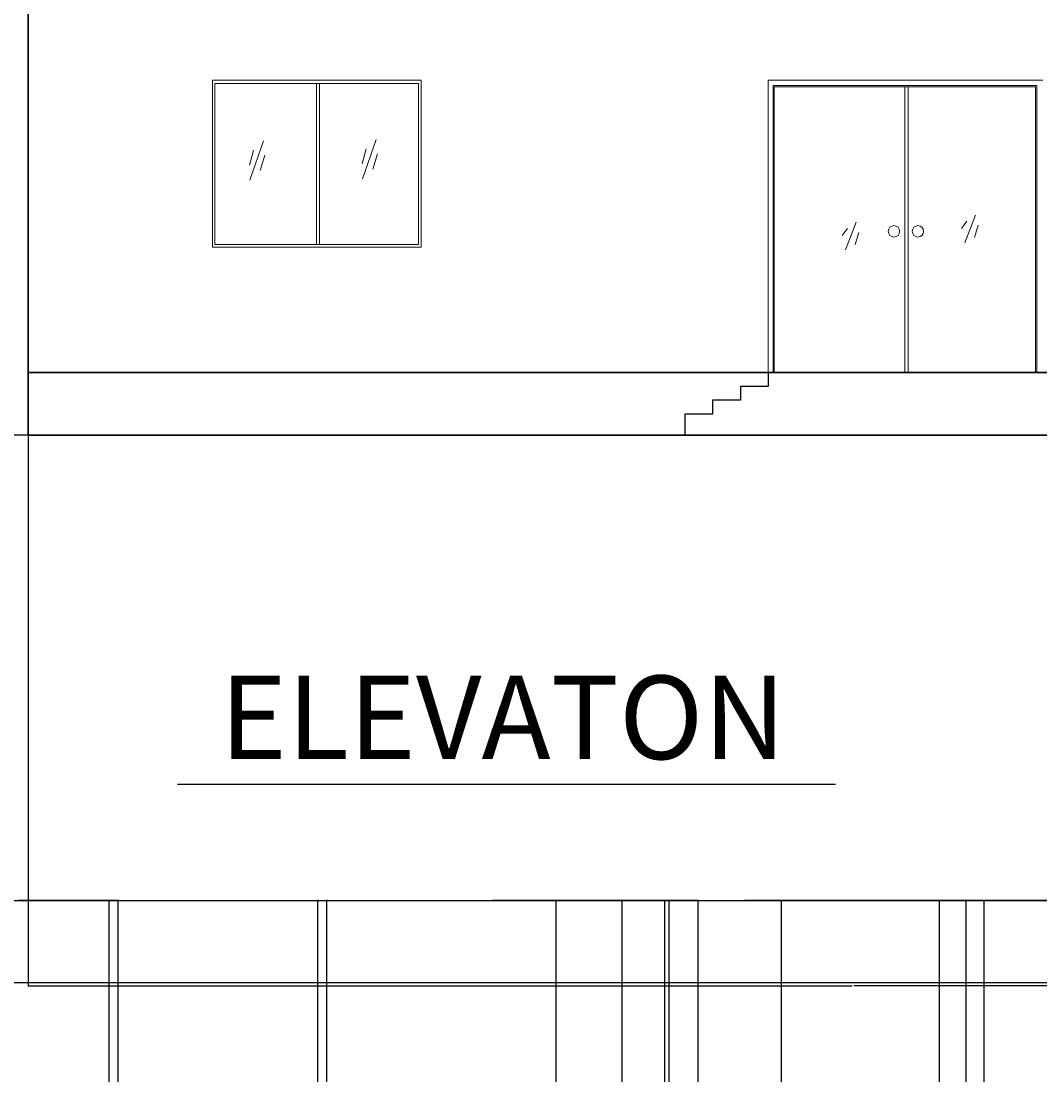
# Model space of a CAD drawing. Units: inches. Extents: x 1770 to 2988, y 1161 to 3221.
# Tile 34 of 44: x 2179 to 2472, y 2520 to 2823. Entities that reach past the tile are written whole.
import ezdxf

# ---------------------------------------------------------------- set-up
doc = ezdxf.new("R2010")
doc.units = ezdxf.units.IN
for name, color, linetype, lineweight in [('A-ANNO-DIMS', 2, 'Continuous', 18), ('A-ANNO-TEXT', 7, 'Continuous', 25), ('A-ANNO-TTLB', 7, 'Continuous', 25), ('A-ELEV', 7, 'Continuous', 35), ('A-ELEV-DOOR', 4, 'Continuous', 18), ('A-ELEV-GLAZ', 4, 'Continuous', 18), ('A-ELEV-STRS', 7, 'Continuous', 25)]:
    doc.layers.add(name, color=color, linetype=linetype, lineweight=lineweight)
doc.styles.get("Standard").update_dxf_attribs({"font": 'arial.ttf'})
doc.dimstyles.get("Standard").update_dxf_attribs({"dimtxt": 0.18, "dimasz": 0.18, "dimexe": 0.18, "dimexo": 0.0625, "dimgap": 0.09, "dimtad": 0, "dimtih": 1, "dimtoh": 1, "dimdec": 4, "dimzin": 0, "dimdsep": 46, "dimtxsty": 'Standard', "dimcen": 0.09, "dimadec": 0, "dimazin": 0, "dimtfac": 1, "dimtdec": 4, "dimtofl": 0, "dimtmove": 0, "dimatfit": 3, "dimfxl": 1, "dimtolj": 1, "dimtzin": 0, "dimarcsym": 0})

# ---------------------------------------------------------------- blocks, each defined once
blk = doc.blocks.new('GLASS-MARK-WINDOW')
for p, q in [((4.02, 11.23), (0.09, 0)), ((1.17, 8.59), (0, 4.27)), ((4.4, 7.13), (3.12, 2.69))]:
    blk.add_line(p, q)
blk = doc.blocks.new('GLASS-MARK-ENTRY')
for p, q in [((1.47, 6.19), (0, 4.09)), ((3.95, 7.93), (0.91, 0)), ((4.77, 5.04), (3.66, 1.5))]:
    blk.add_line(p, q)
blk = doc.blocks.new('*D56')
at = {"layer": 'A-ANNO-DIMS', "color": 0, "lineweight": -2, "transparency": 16777216}
for p, q in [((1971.53, 2506.34), (1971.53, 2570.7)), ((1971.71, 2570.52), (2386.59, 2570.52)), ((2802.26, 2570.52), (2387.38, 2570.52)), ((2802.44, 2506.34), (2802.44, 2570.7))]:
    blk.add_line(p, q, dxfattribs=at)
at = {"layer": 'A-ANNO-DIMS', "color": 0, "transparency": 16777216}
for points in [[(1971.71, 2570.55), (1971.71, 2570.49), (1971.53, 2570.52)], [(2802.26, 2570.55), (2802.26, 2570.49), (2802.44, 2570.52)]]:
    blk.add_solid(points, dxfattribs=at)
at = {"layer": 'Defpoints', "color": 0, "transparency": 16777216}
for p in [(2802.44, 2570.52), (1971.53, 2506.27), (2802.44, 2506.27)]:
    blk.add_point(p, dxfattribs=at)
at = {"layer": 'A-ANNO-DIMS', "color": 0, "transparency": 16777216, "insert": (2386.99, 2570.52), "char_height": 0.18, "attachment_point": 5}
blk.add_mtext('\\A1;830.9', dxfattribs=at)
blk = doc.blocks.new('*D63')
at = {"layer": 'A-ANNO-DIMS', "color": 0, "lineweight": -2, "transparency": 16777216}
for p, q in [((2352.17, 1323.59), (2352.17, 2570.7)), ((2352.35, 2570.52), (2401.24, 2570.52)), ((2450.91, 2570.52), (2402.02, 2570.52)), ((2451.09, 1323.59), (2451.09, 2570.7))]:
    blk.add_line(p, q, dxfattribs=at)
at = {"layer": 'A-ANNO-DIMS', "color": 0, "transparency": 16777216}
for points in [[(2352.35, 2570.55), (2352.35, 2570.49), (2352.17, 2570.52)], [(2450.91, 2570.55), (2450.91, 2570.49), (2451.09, 2570.52)]]:
    blk.add_solid(points, dxfattribs=at)
at = {"layer": 'Defpoints', "color": 0, "transparency": 16777216}
for p in [(2451.09, 2570.52), (2352.17, 1323.53), (2451.09, 1323.53)]:
    blk.add_point(p, dxfattribs=at)
at = {"layer": 'A-ANNO-DIMS', "color": 0, "transparency": 16777216, "insert": (2401.63, 2570.52), "char_height": 0.18, "attachment_point": 5}
blk.add_mtext('\\A1;98.93', dxfattribs=at)
blk = doc.blocks.new('*D64')
at = {"layer": 'A-ANNO-DIMS', "color": 0, "lineweight": -2, "transparency": 16777216}
for p, q in [((2151.7, 2376.76), (2151.7, 2570.7)), ((2151.88, 2570.52), (2179.09, 2570.52)), ((2207.1, 2570.52), (2179.88, 2570.52)), ((2207.28, 2376.76), (2207.28, 2570.7))]:
    blk.add_line(p, q, dxfattribs=at)
at = {"layer": 'A-ANNO-DIMS', "color": 0, "transparency": 16777216}
for points in [[(2151.88, 2570.55), (2151.88, 2570.49), (2151.7, 2570.52)], [(2207.1, 2570.55), (2207.1, 2570.49), (2207.28, 2570.52)]]:
    blk.add_solid(points, dxfattribs=at)
at = {"layer": 'Defpoints', "color": 0, "transparency": 16777216}
for p in [(2207.28, 2570.52), (2151.7, 2376.7), (2207.28, 2376.7)]:
    blk.add_point(p, dxfattribs=at)
at = {"layer": 'A-ANNO-DIMS', "color": 0, "transparency": 16777216, "insert": (2179.49, 2570.52), "char_height": 0.18, "attachment_point": 5}
blk.add_mtext('\\A1;55.58', dxfattribs=at)
blk = doc.blocks.new('*D65')
at = {"layer": 'A-ANNO-DIMS', "color": 0, "lineweight": -2, "transparency": 16777216}
for p, q in [((2267.28, 2376.76), (2267.28, 2570.7)), ((2267.46, 2570.52), (2320.24, 2570.52)), ((2373.79, 2570.52), (2321.01, 2570.52)), ((2373.97, 2376.76), (2373.97, 2570.7))]:
    blk.add_line(p, q, dxfattribs=at)
at = {"layer": 'A-ANNO-DIMS', "color": 0, "transparency": 16777216}
for points in [[(2267.46, 2570.55), (2267.46, 2570.49), (2267.28, 2570.52)], [(2373.79, 2570.55), (2373.79, 2570.49), (2373.97, 2570.52)]]:
    blk.add_solid(points, dxfattribs=at)
at = {"layer": 'Defpoints', "color": 0, "transparency": 16777216}
for p in [(2373.97, 2570.52), (2267.28, 2376.7), (2373.97, 2376.7)]:
    blk.add_point(p, dxfattribs=at)
at = {"layer": 'A-ANNO-DIMS', "color": 0, "transparency": 16777216, "insert": (2320.62, 2570.52), "char_height": 0.18, "attachment_point": 5}
blk.add_mtext('\\A1;106.7', dxfattribs=at)
blk = doc.blocks.new('*D66')
at = {"layer": 'A-ANNO-DIMS', "color": 0, "lineweight": -2, "transparency": 16777216}
for p, q in [((2397.97, 2376.76), (2397.97, 2570.7)), ((2398.15, 2570.52), (2459.91, 2570.52)), ((2522.58, 2570.52), (2460.82, 2570.52)), ((2522.76, 2376.76), (2522.76, 2570.7))]:
    blk.add_line(p, q, dxfattribs=at)
at = {"layer": 'A-ANNO-DIMS', "color": 0, "transparency": 16777216}
for points in [[(2398.15, 2570.55), (2398.15, 2570.49), (2397.97, 2570.52)], [(2522.58, 2570.55), (2522.58, 2570.49), (2522.76, 2570.52)]]:
    blk.add_solid(points, dxfattribs=at)
at = {"layer": 'Defpoints', "color": 0, "transparency": 16777216}
for p in [(2522.76, 2570.52), (2397.97, 2376.7), (2522.76, 2376.7)]:
    blk.add_point(p, dxfattribs=at)
at = {"layer": 'A-ANNO-DIMS', "color": 0, "transparency": 16777216, "insert": (2460.36, 2570.52), "char_height": 0.18, "attachment_point": 5}
blk.add_mtext('\\A1;124.78', dxfattribs=at)
blk = doc.blocks.new('*D68')
at = {"layer": 'A-ANNO-DIMS', "color": 0, "lineweight": -2, "transparency": 16777216}
for p, q in [((2333.2, 2031.76), (2333.2, 2570.7)), ((2333.38, 2570.52), (2394.42, 2570.52)), ((2456.02, 2570.52), (2394.98, 2570.52)), ((2456.2, 2031.76), (2456.2, 2570.7))]:
    blk.add_line(p, q, dxfattribs=at)
at = {"layer": 'A-ANNO-DIMS', "color": 0, "transparency": 16777216}
for points in [[(2333.38, 2570.55), (2333.38, 2570.49), (2333.2, 2570.52)], [(2456.02, 2570.55), (2456.02, 2570.49), (2456.2, 2570.52)]]:
    blk.add_solid(points, dxfattribs=at)
at = {"layer": 'Defpoints', "color": 0, "transparency": 16777216}
for p in [(2456.2, 2570.52), (2333.2, 2031.7), (2456.2, 2031.7)]:
    blk.add_point(p, dxfattribs=at)
at = {"layer": 'A-ANNO-DIMS', "color": 0, "transparency": 16777216, "insert": (2394.7, 2570.52), "char_height": 0.18, "attachment_point": 5}
blk.add_mtext('\\A1;123', dxfattribs=at)
blk = doc.blocks.new('*D79')
at = {"layer": 'A-ANNO-DIMS', "color": 0, "lineweight": -2, "transparency": 16777216}
for p, q in [((2151.7, 1610.26), (2151.7, 2570.7)), ((2151.88, 2570.52), (2177.78, 2570.52)), ((2204.48, 2570.52), (2178.57, 2570.52)), ((2204.66, 1610.26), (2204.66, 2570.7))]:
    blk.add_line(p, q, dxfattribs=at)
at = {"layer": 'A-ANNO-DIMS', "color": 0, "transparency": 16777216}
for points in [[(2151.88, 2570.55), (2151.88, 2570.49), (2151.7, 2570.52)], [(2204.48, 2570.55), (2204.48, 2570.49), (2204.66, 2570.52)]]:
    blk.add_solid(points, dxfattribs=at)
at = {"layer": 'Defpoints', "color": 0, "transparency": 16777216}
for p in [(2204.66, 2570.52), (2151.7, 1610.2), (2204.66, 1610.2)]:
    blk.add_point(p, dxfattribs=at)
at = {"layer": 'A-ANNO-DIMS', "color": 0, "transparency": 16777216, "insert": (2178.18, 2570.52), "char_height": 0.18, "attachment_point": 5}
blk.add_mtext('\\A1;52.96', dxfattribs=at)
blk = doc.blocks.new('*D80')
at = {"layer": 'A-ANNO-DIMS', "color": 0, "lineweight": -2, "transparency": 16777216}
for p, q in [((2264.66, 1610.26), (2264.66, 2570.7)), ((2264.84, 2570.52), (2314.14, 2570.52)), ((2364.23, 2570.52), (2314.93, 2570.52)), ((2364.41, 1610.26), (2364.41, 2570.7))]:
    blk.add_line(p, q, dxfattribs=at)
at = {"layer": 'A-ANNO-DIMS', "color": 0, "transparency": 16777216}
for points in [[(2264.84, 2570.55), (2264.84, 2570.49), (2264.66, 2570.52)], [(2364.23, 2570.55), (2364.23, 2570.49), (2364.41, 2570.52)]]:
    blk.add_solid(points, dxfattribs=at)
at = {"layer": 'Defpoints', "color": 0, "transparency": 16777216}
for p in [(2364.41, 2570.52), (2264.66, 1610.2), (2364.41, 1610.2)]:
    blk.add_point(p, dxfattribs=at)
at = {"layer": 'A-ANNO-DIMS', "color": 0, "transparency": 16777216, "insert": (2314.53, 2570.52), "char_height": 0.18, "attachment_point": 5}
blk.add_mtext('\\A1;99.76', dxfattribs=at)
blk = doc.blocks.new('*D81')
at = {"layer": 'A-ANNO-DIMS', "color": 0, "lineweight": -2, "transparency": 16777216}
for p, q in [((2364.41, 1610.26), (2364.41, 2570.7)), ((2364.59, 2570.52), (2403.51, 2570.52)), ((2443.21, 2570.52), (2404.29, 2570.52)), ((2443.39, 1610.26), (2443.39, 2570.7))]:
    blk.add_line(p, q, dxfattribs=at)
at = {"layer": 'A-ANNO-DIMS', "color": 0, "transparency": 16777216}
for points in [[(2364.59, 2570.55), (2364.59, 2570.49), (2364.41, 2570.52)], [(2443.21, 2570.55), (2443.21, 2570.49), (2443.39, 2570.52)]]:
    blk.add_solid(points, dxfattribs=at)
at = {"layer": 'Defpoints', "color": 0, "transparency": 16777216}
for p in [(2443.39, 2570.52), (2364.41, 1610.2), (2443.39, 1610.2)]:
    blk.add_point(p, dxfattribs=at)
at = {"layer": 'A-ANNO-DIMS', "color": 0, "transparency": 16777216, "insert": (2403.9, 2570.52), "char_height": 0.18, "attachment_point": 5}
blk.add_mtext('\\A1;78.97', dxfattribs=at)
blk = doc.blocks.new('*D82')
at = {"layer": 'A-ANNO-DIMS', "color": 0, "lineweight": -2, "transparency": 16777216}
for p, q in [((2443.39, 1610.26), (2443.39, 2570.7)), ((2443.57, 2570.52), (2486.45, 2570.52)), ((2530.12, 2570.52), (2487.24, 2570.52)), ((2530.3, 1610.26), (2530.3, 2570.7))]:
    blk.add_line(p, q, dxfattribs=at)
at = {"layer": 'A-ANNO-DIMS', "color": 0, "transparency": 16777216}
for points in [[(2443.57, 2570.55), (2443.57, 2570.49), (2443.39, 2570.52)], [(2530.12, 2570.55), (2530.12, 2570.49), (2530.3, 2570.52)]]:
    blk.add_solid(points, dxfattribs=at)
at = {"layer": 'Defpoints', "color": 0, "transparency": 16777216}
for p in [(2530.3, 2570.52), (2443.39, 1610.2), (2530.3, 1610.2)]:
    blk.add_point(p, dxfattribs=at)
at = {"layer": 'A-ANNO-DIMS', "color": 0, "transparency": 16777216, "insert": (2486.85, 2570.52), "char_height": 0.18, "attachment_point": 5}
blk.add_mtext('\\A1;86.92', dxfattribs=at)
blk = doc.blocks.new('*D91')
at = {"layer": 'A-ANNO-DIMS', "color": 0, "lineweight": -2, "transparency": 16777216}
for p, q in [((2333.2, 1839.76), (2333.2, 2570.7)), ((2333.38, 2570.52), (2348.97, 2570.52)), ((2365.49, 2570.52), (2349.9, 2570.52)), ((2365.67, 1839.76), (2365.67, 2570.7))]:
    blk.add_line(p, q, dxfattribs=at)
at = {"layer": 'A-ANNO-DIMS', "color": 0, "transparency": 16777216}
for points in [[(2333.38, 2570.55), (2333.38, 2570.49), (2333.2, 2570.52)], [(2365.49, 2570.55), (2365.49, 2570.49), (2365.67, 2570.52)]]:
    blk.add_solid(points, dxfattribs=at)
at = {"layer": 'Defpoints', "color": 0, "transparency": 16777216}
for p in [(2365.67, 2570.52), (2333.2, 1839.7), (2365.67, 1839.7)]:
    blk.add_point(p, dxfattribs=at)
at = {"layer": 'A-ANNO-DIMS', "color": 0, "transparency": 16777216, "insert": (2349.43, 2570.52), "char_height": 0.18, "attachment_point": 5}
blk.add_mtext('\\A1;32.476', dxfattribs=at)
blk = doc.blocks.new('*D93')
at = {"layer": 'A-ANNO-DIMS', "color": 0, "lineweight": -2, "transparency": 16777216}
for p, q in [((2181.44, 2704.23), (2181.44, 2545.88)), ((2655.44, 2704.23), (2655.44, 2545.88)), ((2181.62, 2546.06), (2418.15, 2546.06)), ((2655.26, 2546.06), (2418.74, 2546.06))]:
    blk.add_line(p, q, dxfattribs=at)
at = {"layer": 'A-ANNO-DIMS', "color": 0, "transparency": 16777216}
for points in [[(2181.62, 2546.09), (2181.62, 2546.03), (2181.44, 2546.06)], [(2655.26, 2546.09), (2655.26, 2546.03), (2655.44, 2546.06)]]:
    blk.add_solid(points, dxfattribs=at)
at = {"layer": 'Defpoints', "color": 0, "transparency": 16777216}
for p in [(2181.44, 2704.3), (2655.44, 2704.3), (2655.44, 2546.06)]:
    blk.add_point(p, dxfattribs=at)
at = {"layer": 'A-ANNO-DIMS', "color": 0, "transparency": 16777216, "insert": (2418.44, 2546.06), "char_height": 0.18, "attachment_point": 5}
blk.add_mtext('\\A1;474', dxfattribs=at)
blk = doc.blocks.new('*D94')
at = {"layer": 'A-ANNO-DIMS', "color": 0, "lineweight": -2, "transparency": 16777216}
for p, q in [((2181.38, 3082.38), (2059.85, 3082.38)), ((2060.03, 3082.2), (2060.03, 2893.52)), ((2060.03, 2704.48), (2060.03, 2893.16)), ((2181.38, 2704.3), (2059.85, 2704.3))]:
    blk.add_line(p, q, dxfattribs=at)
at = {"layer": 'A-ANNO-DIMS', "color": 0, "transparency": 16777216}
for points in [[(2060, 3082.2), (2060.06, 3082.2), (2060.03, 3082.38)], [(2060, 2704.48), (2060.06, 2704.48), (2060.03, 2704.3)]]:
    blk.add_solid(points, dxfattribs=at)
at = {"layer": 'Defpoints', "color": 0, "transparency": 16777216}
for p in [(2060.03, 3082.38), (2181.44, 3082.38), (2181.44, 2704.3)]:
    blk.add_point(p, dxfattribs=at)
at = {"layer": 'A-ANNO-DIMS', "color": 0, "transparency": 16777216, "insert": (2060.03, 2893.34), "char_height": 0.18, "attachment_point": 5}
blk.add_mtext('\\A1;378.1', dxfattribs=at)

msp = doc.modelspace()

# ---------------------------------------------------------------- linework, layer by layer
at = {"layer": 'A-ANNO-TEXT'}
msp.add_line((2224.3288, 2603.9788), (2413.4716, 2603.9788), dxfattribs=at)
at = {"layer": 'A-ANNO-TTLB'}
msp.add_lwpolyline([(2073.6202, 3129.9468), (2769.3644, 3129.9468), (2769.3644, 2546.8952), (2073.6202, 2546.8952)], close=True, dxfattribs=at)
at = {"layer": 'A-ELEV'}
for p, q in [((2181.443, 2890.2969), (2181.443, 2704.2969)), ((2655.443, 2722.2969), (2181.443, 2722.2969)), ((2655.443, 2704.2969), (2181.443, 2704.2969))]:
    msp.add_line(p, q, dxfattribs=at)
at = {"layer": 'A-ELEV-DOOR'}
for p, q in [((2394.1592, 2806.2969), (2394.1592, 2722.2969)), ((2473.1333, 2806.2969), (2394.1592, 2806.2969)), ((2433.4084, 2804.3463), (2433.4084, 2722.2969)), ((2433.4084, 2804.3463), (2434.4084, 2804.3463)), ((2434.4084, 2804.3463), (2434.4084, 2722.2969))]:
    msp.add_line(p, q, dxfattribs=at)
for points in [[(2395.5608, 2804.7493), (2471.3685, 2804.7493), (2471.3685, 2722.2969), (2395.5608, 2722.2969)], [(2395.8833, 2804.3463), (2470.9334, 2804.3463), (2470.9334, 2722.2969), (2395.8833, 2722.2969)]]:
    msp.add_lwpolyline(points, close=True, dxfattribs=at)
for centre in [(2430.297, 2762.8612), (2437.1758, 2762.8612)]:
    msp.add_circle(centre, 1.6332, dxfattribs=at)
at = {"layer": 'A-ELEV-GLAZ'}
for p, q in [((2234.4038, 2806.2969), (2234.4038, 2758.2969)), ((2294.4038, 2806.2969), (2234.4038, 2806.2969)), ((2234.4038, 2806.2969), (2234.4038, 2758.2969)), ((2294.4038, 2806.2969), (2234.4038, 2806.2969)), ((2264.3375, 2805.3181), (2264.3375, 2759.0537)), ((2265.139, 2805.3181), (2265.139, 2759.0537)), ((2294.4038, 2806.2969), (2294.4038, 2758.2969)), ((2294.4038, 2806.2969), (2294.4038, 2758.2969)), ((2294.4038, 2758.2969), (2234.4038, 2758.2969)), ((2294.4038, 2758.2969), (2234.4038, 2758.2969))]:
    msp.add_line(p, q, dxfattribs=at)
msp.add_lwpolyline([(2235.0884, 2805.3181), (2293.5865, 2805.3181), (2293.5865, 2759.0537), (2235.0884, 2759.0537)], close=True, dxfattribs=at)
at = {"layer": 'A-ELEV-STRS'}
for p, q in [((2394.1592, 2722.2969), (2394.1592, 2718.2969)), ((2390.1592, 2718.2969), (2386.1592, 2718.2969)), ((2386.1592, 2718.2969), (2386.1592, 2714.2969)), ((2394.1592, 2718.2969), (2390.1592, 2718.2969)), ((2386.1592, 2714.2969), (2378.1592, 2714.2969)), ((2378.1592, 2714.2969), (2378.1592, 2710.2969)), ((2378.1592, 2710.2969), (2370.1592, 2710.2969)), ((2370.1592, 2710.2969), (2370.1592, 2704.2969))]:
    msp.add_line(p, q, dxfattribs=at)

# ---------------------------------------------------------------- block references
at = {"layer": 'A-ELEV-DOOR'}
for p in [(2415.443, 2757.532), (2449.7466, 2759.5522)]:
    msp.add_blockref('GLASS-MARK-ENTRY', p, dxfattribs=at)
at = {"layer": 'A-ELEV-GLAZ'}
for p in [(2244.9996, 2777.6081), (2277.3808, 2777.9946)]:
    msp.add_blockref('GLASS-MARK-WINDOW', p, dxfattribs=at)

# ---------------------------------------------------------------- texts
at = {"layer": 'A-ANNO-TEXT', "insert": (2236.5336, 2635.1739), "char_height": 24, "attachment_point": 1}
msp.add_mtext_dynamic_manual_height_columns('ELEVATON', width=503.881674, gutter_width=12.5, heights=[0], dxfattribs=at)

# ---------------------------------------------------------------- dimensions: what is measured, and where the dimension line sits
at = {"layer": 'A-ANNO-DIMS'}
dim = msp.add_linear_dim(base=(2060.0309, 3082.3817), p1=(2181.443, 2704.2969), p2=(2181.443, 3082.3817), angle=90, dimstyle='Standard', override={"dimdec": 1, "dimlfac": 1, "dimrnd": 0, "dimzin": 0, "dimdsep": 46, "dimlunit": 2}, dxfattribs=at)
dim.commit()
dim.dimension.update_dxf_attribs({"geometry": '*D94', "text_midpoint": (2060.0309, 2893.3393)})
for base, p1, p2, override, picture, middle in [((2655.443, 2546.0579), (2181.443, 2704.2969), (2655.443, 2704.2969), {"dimdec": 0, "dimlfac": 1, "dimrnd": 0, "dimzin": 0, "dimdsep": 46, "dimlunit": 2}, '*D93', (2418.443, 2546.0579)), ((2802.4374, 2570.5247), (1971.5344, 2506.2747), (2802.4374, 2506.2747), {"dimdec": 1, "dimlfac": 1, "dimrnd": 0, "dimzin": 0, "dimdsep": 46, "dimlunit": 2}, '*D56', (2386.9859, 2570.5247)), ((2207.2776, 2570.5247), (2151.696, 2376.7021), (2207.2776, 2376.7021), {"dimdec": 2, "dimlfac": 1, "dimrnd": 0, "dimzin": 0, "dimdsep": 46, "dimlunit": 2}, '*D64', (2179.4868, 2570.5247)), ((2204.6568, 2570.5247), (2151.696, 1610.2021), (2204.6568, 1610.2021), {"dimdec": 2, "dimlfac": 1, "dimrnd": 0, "dimzin": 0, "dimdsep": 46, "dimlunit": 2}, '*D79', (2178.1764, 2570.5247)), ((2364.4122, 2570.5247), (2264.6568, 1610.2021), (2364.4122, 1610.2021), {"dimdec": 2, "dimlfac": 1, "dimrnd": 0, "dimzin": 0, "dimdsep": 46, "dimlunit": 2}, '*D80', (2314.5345, 2570.5247)), ((2373.9714, 2570.5247), (2267.2776, 2376.7021), (2373.9714, 2376.7021), {"dimdec": 1, "dimlfac": 1, "dimrnd": 0, "dimzin": 0, "dimdsep": 46, "dimlunit": 2}, '*D65', (2320.6245, 2570.5247)), ((2456.196, 2570.5247), (2333.196, 2031.7021), (2456.196, 2031.7021), {"dimdec": 0, "dimlfac": 1, "dimrnd": 0, "dimzin": 0, "dimdsep": 46, "dimlunit": 2}, '*D68', (2394.696, 2570.5247)), ((2365.672, 2570.5247), (2333.196, 1839.7021), (2365.672, 1839.7021), {"dimdec": 3, "dimlfac": 1, "dimrnd": 0, "dimzin": 0, "dimdsep": 46, "dimlunit": 2}, '*D91', (2349.434, 2570.5247)), ((2451.0947, 2570.5247), (2352.1672, 1323.5288), (2451.0947, 1323.5288), {"dimdec": 2, "dimlfac": 1, "dimrnd": 0, "dimzin": 0, "dimdsep": 46, "dimlunit": 2}, '*D63', (2401.631, 2570.5247)), ((2443.3863, 2570.5247), (2364.4122, 1610.2021), (2443.3863, 1610.2021), {"dimdec": 2, "dimlfac": 1, "dimrnd": 0, "dimzin": 0, "dimdsep": 46, "dimlunit": 2}, '*D81', (2403.8993, 2570.5247)), ((2522.7552, 2570.5247), (2397.9714, 2376.7021), (2522.7552, 2376.7021), {"dimdec": 2, "dimlfac": 1, "dimrnd": 0, "dimzin": 0, "dimdsep": 46, "dimlunit": 2}, '*D66', (2460.3633, 2570.5247)), ((2530.3038, 2570.5247), (2443.3863, 1610.2021), (2530.3038, 1610.2021), {"dimdec": 2, "dimlfac": 1, "dimrnd": 0, "dimzin": 0, "dimdsep": 46, "dimlunit": 2}, '*D82', (2486.8451, 2570.5247))]:
    dim = msp.add_linear_dim(base=base, p1=p1, p2=p2, dimstyle='Standard', override=override, dxfattribs=at)
    dim.commit()
    dim.dimension.update_dxf_attribs({"geometry": picture, "text_midpoint": middle})

doc.saveas('drawing.dxf')
